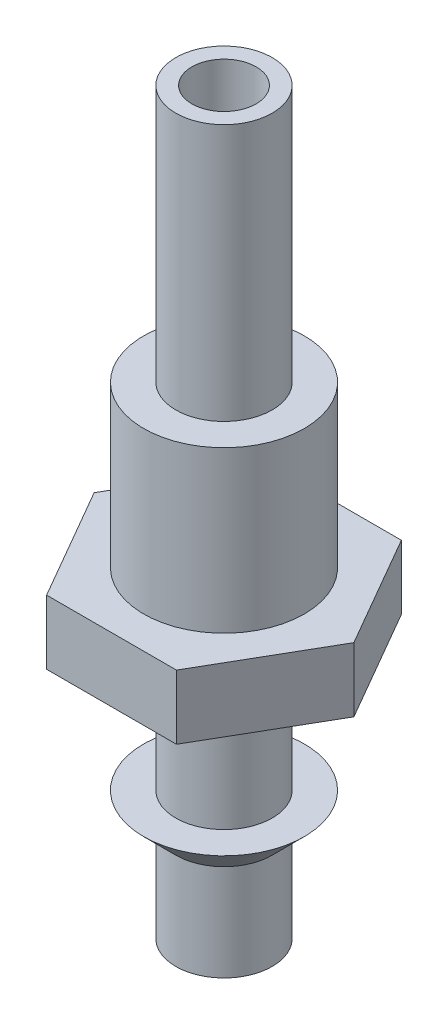
ISO-10303-21;
HEADER;
FILE_DESCRIPTION(('STEP AP214'),'2;1');
FILE_NAME('part.step','',(''),(''),'','','');
FILE_SCHEMA(('AUTOMOTIVE_DESIGN { 1 0 10303 214 1 1 1 1 }'));
ENDSEC;
DATA;
#1=APPLICATION_CONTEXT('core data for automotive mechanical design processes');
#2=APPLICATION_PROTOCOL_DEFINITION('international standard','automotive_design',2000,#1);
#3=PRODUCT_CONTEXT('',#1,'mechanical');
#4=PRODUCT('Part','Part','',(#3));
#5=PRODUCT_RELATED_PRODUCT_CATEGORY('part','',(#4));
#6=PRODUCT_DEFINITION_FORMATION('','',#4);
#7=PRODUCT_DEFINITION_CONTEXT('part definition',#1,'design');
#8=PRODUCT_DEFINITION('design','',#6,#7);
#9=PRODUCT_DEFINITION_SHAPE('','',#8);
#10=(LENGTH_UNIT() NAMED_UNIT(*) SI_UNIT(.MILLI.,.METRE.));
#11=(NAMED_UNIT(*) PLANE_ANGLE_UNIT() SI_UNIT($,.RADIAN.));
#12=(NAMED_UNIT(*) SI_UNIT($,.STERADIAN.) SOLID_ANGLE_UNIT());
#13=UNCERTAINTY_MEASURE_WITH_UNIT(LENGTH_MEASURE(1.E-05),#10,'distance_accuracy_value','');
#14=(GEOMETRIC_REPRESENTATION_CONTEXT(3) GLOBAL_UNCERTAINTY_ASSIGNED_CONTEXT((#13)) GLOBAL_UNIT_ASSIGNED_CONTEXT((#10,
#11,#12)) REPRESENTATION_CONTEXT('',''));
#15=CARTESIAN_POINT('',(0.,0.,0.));
#16=DIRECTION('',(0.,0.,1.));
#17=DIRECTION('',(1.,0.,0.));
#18=AXIS2_PLACEMENT_3D('',#15,#16,#17);
#19=CARTESIAN_POINT('',(0.,-8.,0.));
#20=DIRECTION('',(0.,1.,0.));
#21=DIRECTION('',(0.,0.,1.));
#22=AXIS2_PLACEMENT_3D('',#19,#20,#21);
#23=PLANE('',#22);
#24=CARTESIAN_POINT('',(0.,-8.,0.));
#25=DIRECTION('',(0.,1.,0.));
#26=DIRECTION('',(-1.,0.,0.));
#27=AXIS2_PLACEMENT_3D('',#24,#25,#26);
#28=CIRCLE('',#27,1.);
#29=CARTESIAN_POINT('',(-0.999999999999999,-8.,0.));
#30=VERTEX_POINT('',#29);
#31=EDGE_CURVE('E168',#30,#30,#28,.T.);
#32=ORIENTED_EDGE('',*,*,#31,.T.);
#33=EDGE_LOOP('',(#32));
#34=FACE_BOUND('',#33,.T.);
#35=CARTESIAN_POINT('',(0.,-8.,0.));
#36=DIRECTION('',(0.,1.,0.));
#37=DIRECTION('',(0.,0.,1.));
#38=AXIS2_PLACEMENT_3D('',#35,#36,#37);
#39=CIRCLE('',#38,1.5);
#40=CARTESIAN_POINT('',(0.,-8.,1.5));
#41=VERTEX_POINT('',#40);
#42=EDGE_CURVE('E11',#41,#41,#39,.T.);
#43=ORIENTED_EDGE('',*,*,#42,.F.);
#44=EDGE_LOOP('',(#43));
#45=FACE_BOUND('',#44,.T.);
#46=ADVANCED_FACE('F39',(#34,#45),#23,.F.);
#47=CARTESIAN_POINT('',(0.,0.,0.));
#48=DIRECTION('',(0.,1.,0.));
#49=DIRECTION('',(0.,0.,1.));
#50=AXIS2_PLACEMENT_3D('',#47,#48,#49);
#51=CYLINDRICAL_SURFACE('',#50,1.5);
#52=CARTESIAN_POINT('',(0.,-5.,0.));
#53=DIRECTION('',(0.,1.,0.));
#54=DIRECTION('',(0.,0.,1.));
#55=AXIS2_PLACEMENT_3D('',#52,#53,#54);
#56=CIRCLE('',#55,1.5);
#57=CARTESIAN_POINT('',(0.,-5.,1.5));
#58=VERTEX_POINT('',#57);
#59=EDGE_CURVE('E50',#58,#58,#56,.T.);
#60=ORIENTED_EDGE('',*,*,#59,.F.);
#61=EDGE_LOOP('',(#60));
#62=FACE_BOUND('',#61,.T.);
#63=ORIENTED_EDGE('',*,*,#42,.T.);
#64=EDGE_LOOP('',(#63));
#65=FACE_BOUND('',#64,.T.);
#66=ADVANCED_FACE('F160',(#62,#65),#51,.T.);
#67=CARTESIAN_POINT('',(0.,-5.,0.));
#68=DIRECTION('',(0.,1.,0.));
#69=DIRECTION('',(0.,0.,1.));
#70=AXIS2_PLACEMENT_3D('',#67,#68,#69);
#71=CONICAL_SURFACE('',#70,1.5,0.785398163397448);
#72=CARTESIAN_POINT('',(0.,-4.,0.));
#73=DIRECTION('',(0.,1.,0.));
#74=DIRECTION('',(0.,0.,1.));
#75=AXIS2_PLACEMENT_3D('',#72,#73,#74);
#76=CIRCLE('',#75,2.5);
#77=CARTESIAN_POINT('',(0.,-4.,2.5));
#78=VERTEX_POINT('',#77);
#79=EDGE_CURVE('E147',#78,#78,#76,.T.);
#80=ORIENTED_EDGE('',*,*,#79,.F.);
#81=EDGE_LOOP('',(#80));
#82=FACE_BOUND('',#81,.T.);
#83=ORIENTED_EDGE('',*,*,#59,.T.);
#84=EDGE_LOOP('',(#83));
#85=FACE_BOUND('',#84,.T.);
#86=ADVANCED_FACE('F154',(#82,#85),#71,.T.);
#87=CARTESIAN_POINT('',(2.5,-4.,0.));
#88=DIRECTION('',(0.,-1.,0.));
#89=DIRECTION('',(0.,0.,-1.));
#90=AXIS2_PLACEMENT_3D('',#87,#88,#89);
#91=PLANE('',#90);
#92=CARTESIAN_POINT('',(0.,-4.,0.));
#93=DIRECTION('',(0.,1.,0.));
#94=DIRECTION('',(0.,0.,1.));
#95=AXIS2_PLACEMENT_3D('',#92,#93,#94);
#96=CIRCLE('',#95,1.50000000000003);
#97=CARTESIAN_POINT('',(0.,-4.,1.50000000000003));
#98=VERTEX_POINT('',#97);
#99=EDGE_CURVE('E150',#98,#98,#96,.T.);
#100=ORIENTED_EDGE('',*,*,#99,.F.);
#101=EDGE_LOOP('',(#100));
#102=FACE_BOUND('',#101,.T.);
#103=ORIENTED_EDGE('',*,*,#79,.T.);
#104=EDGE_LOOP('',(#103));
#105=FACE_BOUND('',#104,.T.);
#106=ADVANCED_FACE('F221',(#102,#105),#91,.F.);
#107=CARTESIAN_POINT('',(0.,0.,0.));
#108=DIRECTION('',(0.,1.,0.));
#109=DIRECTION('',(0.,0.,1.));
#110=AXIS2_PLACEMENT_3D('',#107,#108,#109);
#111=CYLINDRICAL_SURFACE('',#110,1.50000000000003);
#112=CARTESIAN_POINT('',(0.,0.,0.));
#113=DIRECTION('',(0.,1.,0.));
#114=DIRECTION('',(0.,0.,1.));
#115=AXIS2_PLACEMENT_3D('',#112,#113,#114);
#116=CIRCLE('',#115,1.50000000000003);
#117=CARTESIAN_POINT('',(0.,0.,1.50000000000003));
#118=VERTEX_POINT('',#117);
#119=EDGE_CURVE('E145',#118,#118,#116,.T.);
#120=ORIENTED_EDGE('',*,*,#119,.F.);
#121=EDGE_LOOP('',(#120));
#122=FACE_BOUND('',#121,.T.);
#123=ORIENTED_EDGE('',*,*,#99,.T.);
#124=EDGE_LOOP('',(#123));
#125=FACE_BOUND('',#124,.T.);
#126=ADVANCED_FACE('F222',(#122,#125),#111,.T.);
#127=CARTESIAN_POINT('',(2.02072594216369,2.,3.5));
#128=DIRECTION('',(-0.866025403784439,0.,-0.5));
#129=DIRECTION('',(-0.5,0.,0.866025403784439));
#130=AXIS2_PLACEMENT_3D('',#127,#128,#129);
#131=PLANE('',#130);
#132=DIRECTION('',(0.5,0.,-0.866025403784439));
#133=VECTOR('',#132,1.);
#134=CARTESIAN_POINT('',(2.02072594216369,0.,3.5));
#135=LINE('',#134,#133);
#136=CARTESIAN_POINT('',(2.02072594216369,0.,3.5));
#137=VERTEX_POINT('',#136);
#138=CARTESIAN_POINT('',(4.04145188432738,0.,0.));
#139=VERTEX_POINT('',#138);
#140=EDGE_CURVE('E121',#137,#139,#135,.T.);
#141=ORIENTED_EDGE('',*,*,#140,.T.);
#142=DIRECTION('',(0.,-1.,0.));
#143=VECTOR('',#142,1.);
#144=CARTESIAN_POINT('',(4.04145188432738,2.,0.));
#145=LINE('',#144,#143);
#146=CARTESIAN_POINT('',(4.04145188432738,2.,0.));
#147=VERTEX_POINT('',#146);
#148=EDGE_CURVE('E142',#147,#139,#145,.T.);
#149=ORIENTED_EDGE('',*,*,#148,.F.);
#150=DIRECTION('',(0.5,0.,-0.866025403784439));
#151=VECTOR('',#150,1.);
#152=CARTESIAN_POINT('',(2.02072594216369,2.,3.5));
#153=LINE('',#152,#151);
#154=CARTESIAN_POINT('',(2.02072594216369,2.,3.5));
#155=VERTEX_POINT('',#154);
#156=EDGE_CURVE('E131',#155,#147,#153,.T.);
#157=ORIENTED_EDGE('',*,*,#156,.F.);
#158=DIRECTION('',(0.,-1.,0.));
#159=VECTOR('',#158,1.);
#160=CARTESIAN_POINT('',(2.02072594216369,2.,3.5));
#161=LINE('',#160,#159);
#162=EDGE_CURVE('E116',#155,#137,#161,.T.);
#163=ORIENTED_EDGE('',*,*,#162,.T.);
#164=EDGE_LOOP('',(#141,#149,#157,#163));
#165=FACE_BOUND('',#164,.T.);
#166=ADVANCED_FACE('F200',(#165),#131,.F.);
#167=CARTESIAN_POINT('',(4.04145188432738,2.,0.));
#168=DIRECTION('',(-0.866025403784438,0.,0.5));
#169=DIRECTION('',(0.5,0.,0.866025403784439));
#170=AXIS2_PLACEMENT_3D('',#167,#168,#169);
#171=PLANE('',#170);
#172=DIRECTION('',(-0.5,0.,-0.866025403784438));
#173=VECTOR('',#172,1.);
#174=CARTESIAN_POINT('',(4.04145188432738,0.,0.));
#175=LINE('',#174,#173);
#176=CARTESIAN_POINT('',(2.02072594216369,0.,-3.5));
#177=VERTEX_POINT('',#176);
#178=EDGE_CURVE('E130',#139,#177,#175,.T.);
#179=ORIENTED_EDGE('',*,*,#178,.T.);
#180=DIRECTION('',(0.,-1.,0.));
#181=VECTOR('',#180,1.);
#182=CARTESIAN_POINT('',(2.02072594216369,2.,-3.5));
#183=LINE('',#182,#181);
#184=CARTESIAN_POINT('',(2.02072594216369,2.,-3.5));
#185=VERTEX_POINT('',#184);
#186=EDGE_CURVE('E136',#185,#177,#183,.T.);
#187=ORIENTED_EDGE('',*,*,#186,.F.);
#188=DIRECTION('',(-0.5,0.,-0.866025403784438));
#189=VECTOR('',#188,1.);
#190=CARTESIAN_POINT('',(4.04145188432738,2.,0.));
#191=LINE('',#190,#189);
#192=EDGE_CURVE('E91',#147,#185,#191,.T.);
#193=ORIENTED_EDGE('',*,*,#192,.F.);
#194=ORIENTED_EDGE('',*,*,#148,.T.);
#195=EDGE_LOOP('',(#179,#187,#193,#194));
#196=FACE_BOUND('',#195,.T.);
#197=ADVANCED_FACE('F192',(#196),#171,.F.);
#198=CARTESIAN_POINT('',(2.02072594216369,2.,-3.5));
#199=DIRECTION('',(0.,0.,1.));
#200=DIRECTION('',(1.,0.,0.));
#201=AXIS2_PLACEMENT_3D('',#198,#199,#200);
#202=PLANE('',#201);
#203=DIRECTION('',(-1.,0.,0.));
#204=VECTOR('',#203,1.);
#205=CARTESIAN_POINT('',(2.02072594216369,0.,-3.5));
#206=LINE('',#205,#204);
#207=CARTESIAN_POINT('',(-2.02072594216369,0.,-3.5));
#208=VERTEX_POINT('',#207);
#209=EDGE_CURVE('E128',#177,#208,#206,.T.);
#210=ORIENTED_EDGE('',*,*,#209,.T.);
#211=DIRECTION('',(0.,-1.,0.));
#212=VECTOR('',#211,1.);
#213=CARTESIAN_POINT('',(-2.02072594216369,2.,-3.5));
#214=LINE('',#213,#212);
#215=CARTESIAN_POINT('',(-2.02072594216369,2.,-3.5));
#216=VERTEX_POINT('',#215);
#217=EDGE_CURVE('E113',#216,#208,#214,.T.);
#218=ORIENTED_EDGE('',*,*,#217,.F.);
#219=DIRECTION('',(-1.,0.,0.));
#220=VECTOR('',#219,1.);
#221=CARTESIAN_POINT('',(2.02072594216369,2.,-3.5));
#222=LINE('',#221,#220);
#223=EDGE_CURVE('E106',#185,#216,#222,.T.);
#224=ORIENTED_EDGE('',*,*,#223,.F.);
#225=ORIENTED_EDGE('',*,*,#186,.T.);
#226=EDGE_LOOP('',(#210,#218,#224,#225));
#227=FACE_BOUND('',#226,.T.);
#228=ADVANCED_FACE('F191',(#227),#202,.F.);
#229=CARTESIAN_POINT('',(-2.02072594216369,2.,-3.5));
#230=DIRECTION('',(0.866025403784439,0.,0.5));
#231=DIRECTION('',(0.5,0.,-0.866025403784439));
#232=AXIS2_PLACEMENT_3D('',#229,#230,#231);
#233=PLANE('',#232);
#234=DIRECTION('',(-0.5,0.,0.866025403784439));
#235=VECTOR('',#234,1.);
#236=CARTESIAN_POINT('',(-2.02072594216369,0.,-3.5));
#237=LINE('',#236,#235);
#238=CARTESIAN_POINT('',(-4.04145188432738,0.,0.));
#239=VERTEX_POINT('',#238);
#240=EDGE_CURVE('E111',#208,#239,#237,.T.);
#241=ORIENTED_EDGE('',*,*,#240,.T.);
#242=DIRECTION('',(0.,-1.,0.));
#243=VECTOR('',#242,1.);
#244=CARTESIAN_POINT('',(-4.04145188432738,2.,0.));
#245=LINE('',#244,#243);
#246=CARTESIAN_POINT('',(-4.04145188432738,2.,0.));
#247=VERTEX_POINT('',#246);
#248=EDGE_CURVE('E112',#247,#239,#245,.T.);
#249=ORIENTED_EDGE('',*,*,#248,.F.);
#250=DIRECTION('',(-0.5,0.,0.866025403784439));
#251=VECTOR('',#250,1.);
#252=CARTESIAN_POINT('',(-2.02072594216369,2.,-3.5));
#253=LINE('',#252,#251);
#254=EDGE_CURVE('E99',#216,#247,#253,.T.);
#255=ORIENTED_EDGE('',*,*,#254,.F.);
#256=ORIENTED_EDGE('',*,*,#217,.T.);
#257=EDGE_LOOP('',(#241,#249,#255,#256));
#258=FACE_BOUND('',#257,.T.);
#259=ADVANCED_FACE('F115',(#258),#233,.F.);
#260=CARTESIAN_POINT('',(-4.04145188432738,2.,0.));
#261=DIRECTION('',(0.866025403784438,0.,-0.5));
#262=DIRECTION('',(-0.5,0.,-0.866025403784438));
#263=AXIS2_PLACEMENT_3D('',#260,#261,#262);
#264=PLANE('',#263);
#265=DIRECTION('',(0.5,0.,0.866025403784438));
#266=VECTOR('',#265,1.);
#267=CARTESIAN_POINT('',(-4.04145188432738,0.,0.));
#268=LINE('',#267,#266);
#269=CARTESIAN_POINT('',(-2.02072594216369,0.,3.5));
#270=VERTEX_POINT('',#269);
#271=EDGE_CURVE('E77',#239,#270,#268,.T.);
#272=ORIENTED_EDGE('',*,*,#271,.T.);
#273=DIRECTION('',(0.,-1.,0.));
#274=VECTOR('',#273,1.);
#275=CARTESIAN_POINT('',(-2.02072594216369,2.,3.5));
#276=LINE('',#275,#274);
#277=CARTESIAN_POINT('',(-2.02072594216369,2.,3.5));
#278=VERTEX_POINT('',#277);
#279=EDGE_CURVE('E118',#278,#270,#276,.T.);
#280=ORIENTED_EDGE('',*,*,#279,.F.);
#281=DIRECTION('',(0.5,0.,0.866025403784438));
#282=VECTOR('',#281,1.);
#283=CARTESIAN_POINT('',(-4.04145188432738,2.,0.));
#284=LINE('',#283,#282);
#285=EDGE_CURVE('E102',#247,#278,#284,.T.);
#286=ORIENTED_EDGE('',*,*,#285,.F.);
#287=ORIENTED_EDGE('',*,*,#248,.T.);
#288=EDGE_LOOP('',(#272,#280,#286,#287));
#289=FACE_BOUND('',#288,.T.);
#290=ADVANCED_FACE('F117',(#289),#264,.F.);
#291=CARTESIAN_POINT('',(-2.02072594216369,2.,3.5));
#292=DIRECTION('',(0.,0.,-1.));
#293=DIRECTION('',(-1.,0.,0.));
#294=AXIS2_PLACEMENT_3D('',#291,#292,#293);
#295=PLANE('',#294);
#296=DIRECTION('',(1.,0.,0.));
#297=VECTOR('',#296,1.);
#298=CARTESIAN_POINT('',(-2.02072594216369,0.,3.5));
#299=LINE('',#298,#297);
#300=EDGE_CURVE('E81',#270,#137,#299,.T.);
#301=ORIENTED_EDGE('',*,*,#300,.T.);
#302=ORIENTED_EDGE('',*,*,#162,.F.);
#303=DIRECTION('',(1.,0.,0.));
#304=VECTOR('',#303,1.);
#305=CARTESIAN_POINT('',(-2.02072594216369,2.,3.5));
#306=LINE('',#305,#304);
#307=EDGE_CURVE('E54',#278,#155,#306,.T.);
#308=ORIENTED_EDGE('',*,*,#307,.F.);
#309=ORIENTED_EDGE('',*,*,#279,.T.);
#310=EDGE_LOOP('',(#301,#302,#308,#309));
#311=FACE_BOUND('',#310,.T.);
#312=ADVANCED_FACE('F199',(#311),#295,.F.);
#313=CARTESIAN_POINT('',(0.,2.,0.));
#314=DIRECTION('',(0.,1.,0.));
#315=DIRECTION('',(0.,0.,1.));
#316=AXIS2_PLACEMENT_3D('',#313,#314,#315);
#317=PLANE('',#316);
#318=CARTESIAN_POINT('',(0.,2.,0.));
#319=DIRECTION('',(0.,-1.,0.));
#320=DIRECTION('',(1.,0.,0.));
#321=AXIS2_PLACEMENT_3D('',#318,#319,#320);
#322=CIRCLE('',#321,2.5);
#323=CARTESIAN_POINT('',(2.5,2.,0.));
#324=VERTEX_POINT('',#323);
#325=EDGE_CURVE('E174',#324,#324,#322,.T.);
#326=ORIENTED_EDGE('',*,*,#325,.T.);
#327=EDGE_LOOP('',(#326));
#328=FACE_BOUND('',#327,.T.);
#329=ORIENTED_EDGE('',*,*,#156,.T.);
#330=ORIENTED_EDGE('',*,*,#192,.T.);
#331=ORIENTED_EDGE('',*,*,#223,.T.);
#332=ORIENTED_EDGE('',*,*,#254,.T.);
#333=ORIENTED_EDGE('',*,*,#285,.T.);
#334=ORIENTED_EDGE('',*,*,#307,.T.);
#335=EDGE_LOOP('',(#329,#330,#331,#332,#333,#334));
#336=FACE_BOUND('',#335,.T.);
#337=ADVANCED_FACE('F105',(#328,#336),#317,.T.);
#338=CARTESIAN_POINT('',(0.,0.,0.));
#339=DIRECTION('',(0.,1.,0.));
#340=DIRECTION('',(0.,0.,1.));
#341=AXIS2_PLACEMENT_3D('',#338,#339,#340);
#342=PLANE('',#341);
#343=ORIENTED_EDGE('',*,*,#119,.T.);
#344=EDGE_LOOP('',(#343));
#345=FACE_BOUND('',#344,.T.);
#346=ORIENTED_EDGE('',*,*,#140,.F.);
#347=ORIENTED_EDGE('',*,*,#300,.F.);
#348=ORIENTED_EDGE('',*,*,#271,.F.);
#349=ORIENTED_EDGE('',*,*,#240,.F.);
#350=ORIENTED_EDGE('',*,*,#209,.F.);
#351=ORIENTED_EDGE('',*,*,#178,.F.);
#352=EDGE_LOOP('',(#346,#347,#348,#349,#350,#351));
#353=FACE_BOUND('',#352,.T.);
#354=ADVANCED_FACE('F197',(#345,#353),#342,.F.);
#355=CARTESIAN_POINT('',(0.,15.,0.));
#356=DIRECTION('',(0.,1.,0.));
#357=DIRECTION('',(-1.,0.,0.));
#358=AXIS2_PLACEMENT_3D('',#355,#356,#357);
#359=PLANE('',#358);
#360=CARTESIAN_POINT('',(0.,15.,0.));
#361=DIRECTION('',(0.,1.,0.));
#362=DIRECTION('',(-1.,0.,0.));
#363=AXIS2_PLACEMENT_3D('',#360,#361,#362);
#364=CIRCLE('',#363,1.);
#365=CARTESIAN_POINT('',(-1.,15.,0.));
#366=VERTEX_POINT('',#365);
#367=EDGE_CURVE('E172',#366,#366,#364,.T.);
#368=ORIENTED_EDGE('',*,*,#367,.F.);
#369=EDGE_LOOP('',(#368));
#370=FACE_BOUND('',#369,.T.);
#371=CARTESIAN_POINT('',(0.,15.,0.));
#372=DIRECTION('',(0.,-1.,0.));
#373=DIRECTION('',(1.,0.,0.));
#374=AXIS2_PLACEMENT_3D('',#371,#372,#373);
#375=CIRCLE('',#374,1.5);
#376=CARTESIAN_POINT('',(1.5,15.,0.));
#377=VERTEX_POINT('',#376);
#378=EDGE_CURVE('E126',#377,#377,#375,.T.);
#379=ORIENTED_EDGE('',*,*,#378,.F.);
#380=EDGE_LOOP('',(#379));
#381=FACE_BOUND('',#380,.T.);
#382=ADVANCED_FACE('F295',(#370,#381),#359,.T.);
#383=CARTESIAN_POINT('',(0.,2.,0.));
#384=DIRECTION('',(0.,-1.,0.));
#385=DIRECTION('',(1.,0.,0.));
#386=AXIS2_PLACEMENT_3D('',#383,#384,#385);
#387=CYLINDRICAL_SURFACE('',#386,1.5);
#388=ORIENTED_EDGE('',*,*,#378,.T.);
#389=EDGE_LOOP('',(#388));
#390=FACE_BOUND('',#389,.T.);
#391=CARTESIAN_POINT('',(0.,7.,0.));
#392=DIRECTION('',(0.,-1.,0.));
#393=DIRECTION('',(1.,0.,0.));
#394=AXIS2_PLACEMENT_3D('',#391,#392,#393);
#395=CIRCLE('',#394,1.5);
#396=CARTESIAN_POINT('',(1.5,7.,0.));
#397=VERTEX_POINT('',#396);
#398=EDGE_CURVE('E181',#397,#397,#395,.T.);
#399=ORIENTED_EDGE('',*,*,#398,.F.);
#400=EDGE_LOOP('',(#399));
#401=FACE_BOUND('',#400,.T.);
#402=ADVANCED_FACE('F296',(#390,#401),#387,.T.);
#403=CARTESIAN_POINT('',(1.5,7.,0.));
#404=DIRECTION('',(0.,1.,0.));
#405=DIRECTION('',(-1.,0.,0.));
#406=AXIS2_PLACEMENT_3D('',#403,#404,#405);
#407=PLANE('',#406);
#408=ORIENTED_EDGE('',*,*,#398,.T.);
#409=EDGE_LOOP('',(#408));
#410=FACE_BOUND('',#409,.T.);
#411=CARTESIAN_POINT('',(0.,7.,0.));
#412=DIRECTION('',(0.,-1.,0.));
#413=DIRECTION('',(1.,0.,0.));
#414=AXIS2_PLACEMENT_3D('',#411,#412,#413);
#415=CIRCLE('',#414,2.5);
#416=CARTESIAN_POINT('',(2.5,7.,0.));
#417=VERTEX_POINT('',#416);
#418=EDGE_CURVE('E177',#417,#417,#415,.T.);
#419=ORIENTED_EDGE('',*,*,#418,.F.);
#420=EDGE_LOOP('',(#419));
#421=FACE_BOUND('',#420,.T.);
#422=ADVANCED_FACE('F309',(#410,#421),#407,.T.);
#423=CARTESIAN_POINT('',(0.,2.,0.));
#424=DIRECTION('',(0.,-1.,0.));
#425=DIRECTION('',(1.,0.,0.));
#426=AXIS2_PLACEMENT_3D('',#423,#424,#425);
#427=CYLINDRICAL_SURFACE('',#426,2.5);
#428=ORIENTED_EDGE('',*,*,#418,.T.);
#429=EDGE_LOOP('',(#428));
#430=FACE_BOUND('',#429,.T.);
#431=ORIENTED_EDGE('',*,*,#325,.F.);
#432=EDGE_LOOP('',(#431));
#433=FACE_BOUND('',#432,.T.);
#434=ADVANCED_FACE('F319',(#430,#433),#427,.T.);
#435=CARTESIAN_POINT('',(0.,-8.,0.));
#436=DIRECTION('',(0.,1.,0.));
#437=DIRECTION('',(-1.,0.,0.));
#438=AXIS2_PLACEMENT_3D('',#435,#436,#437);
#439=CYLINDRICAL_SURFACE('',#438,1.);
#440=ORIENTED_EDGE('',*,*,#31,.F.);
#441=EDGE_LOOP('',(#440));
#442=FACE_BOUND('',#441,.T.);
#443=ORIENTED_EDGE('',*,*,#367,.T.);
#444=EDGE_LOOP('',(#443));
#445=FACE_BOUND('',#444,.T.);
#446=ADVANCED_FACE('F328',(#442,#445),#439,.F.);
#447=CLOSED_SHELL('',(#46,#66,#86,#106,#126,#166,#197,#228,#259,#290,#312,#337,#354,#382,#402,
#422,#434,#446));
#448=MANIFOLD_SOLID_BREP('B2',#447);
#449=ADVANCED_BREP_SHAPE_REPRESENTATION('',(#18,#448),#14);
#450=SHAPE_DEFINITION_REPRESENTATION(#9,#449);
ENDSEC;
END-ISO-10303-21;
